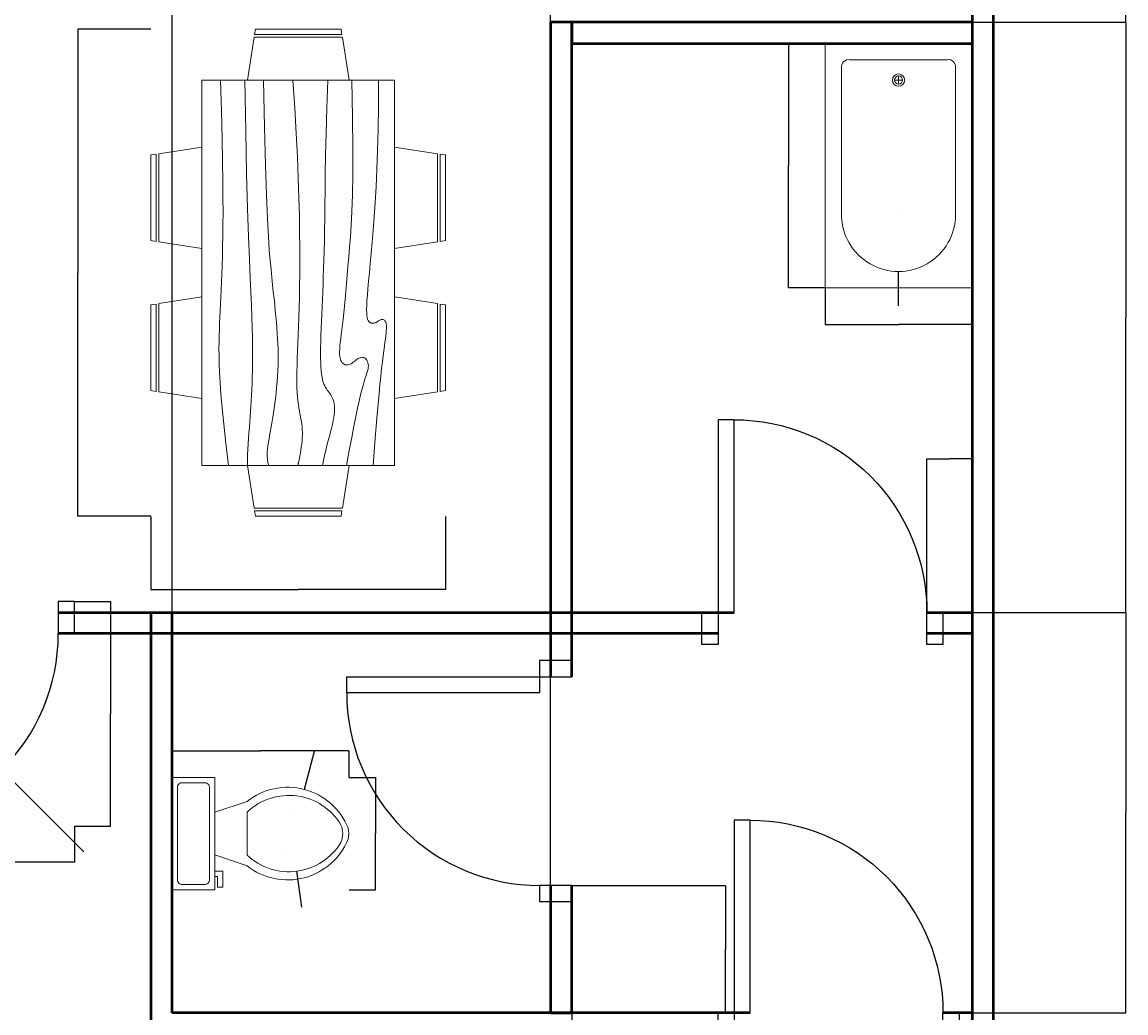
# Model space of a CAD drawing. Units: millimetres. Extents: x 756 to 17937, y 31 to 15590.
# Tile 4 of 6: x 7469 to 12704, y 7660 to 12361. Entities that reach past the tile are written whole.
import ezdxf

# ---------------------------------------------------------------- set-up
doc = ezdxf.new("R2010")
doc.units = ezdxf.units.MM
for name, color, linetype, lineweight in [('A-ANNO-DIMS', 2, 'Continuous', 18), ('A-DOOR', 3, 'Continuous', 25), ('A-FLOR-FIXT', 9, 'Continuous', 18), ('A-FURN', 8, 'Continuous', 18), ('A-WALL', 7, 'Continuous', 50)]:
    doc.layers.add(name, color=color, linetype=linetype, lineweight=lineweight)
doc.styles.get("Standard").update_dxf_attribs({"font": 'arial.ttf'})
doc.dimstyles.get("Standard").update_dxf_attribs({"dimtxt": 0.18, "dimasz": 0.18, "dimexe": 0.18, "dimexo": 0.0625, "dimgap": 0.09, "dimtad": 0, "dimtih": 1, "dimtoh": 1, "dimdec": 4, "dimzin": 0, "dimdsep": 46, "dimtxsty": 'Standard', "dimcen": 0.09, "dimadec": 0, "dimazin": 0, "dimtfac": 1, "dimtdec": 4, "dimtofl": 0, "dimtmove": 0, "dimatfit": 3, "dimfxl": 1, "dimtolj": 1, "dimtzin": 0, "dimarcsym": 0})

# ---------------------------------------------------------------- blocks, each defined once
blk = doc.blocks.new('Dining Set - 36 x 72 in.')
for p, q in [((-22, 27.5), (-22.1562, 26.50042)), ((-22, 27.5), (-6, 27.5)), ((-5.8437, 26.49966), (-6, 27.5)), ((6, 27.5), (5.8438, 26.50042)), ((6, 27.5), (22, 27.5)), ((22.1563, 26.49966), (22, 27.5)), ((-22.2343, 26.00059), (-23.4847, 17.99762)), ((-22.2304, 26), (-5.7608, 26)), ((-5.8416, 26.5), (-22.1534, 26.5)), ((-4.5152, 17.99762), (-5.7655, 25.99926)), ((5.7657, 26.00059), (4.5153, 17.99762)), ((5.7696, 26), (22.2392, 26)), ((22.1584, 26.5), (5.8466, 26.5)), ((23.4848, 17.99762), (22.2345, 25.99926)), ((36, 18), (-36, 18)), ((-36, 18), (-36, -18)), ((36, -18), (36, 18)), ((-44.0006, 8.23428), (-35.9976, 9.48474)), ((44.0006, 8.23428), (35.9976, 9.48474)), ((-45.5, 8), (-44.5004, 8.15617)), ((-45.5, 8), (-45.5, -8)), ((-44.5, -8.15843), (-44.5, 8.15338)), ((-44, 8.23041), (-44, -8.23915)), ((44, 8.23041), (44, -8.23915)), ((44.5, -8.15843), (44.5, 8.15338)), ((45.5, 8), (44.5005, 8.15617)), ((45.5, 8), (45.5, -8)), ((-44.4997, -8.15631), (-45.5, -8)), ((-35.9976, -9.48476), (-43.9993, -8.2345)), ((35.9976, -9.48476), (43.9993, -8.2345)), ((44.4997, -8.15631), (45.5, -8)), ((-36, -18), (36, -18)), ((-22.2343, -26.0006), (-23.4847, -17.99762)), ((-4.5152, -17.99762), (-5.7655, -25.99928)), ((5.7657, -26.0006), (4.5153, -17.99762)), ((23.4848, -17.99762), (22.2345, -25.99928)), ((-22.2304, -26), (-5.7608, -26)), ((-22, -27.5), (-22.1562, -26.50044)), ((-5.8416, -26.5), (-22.1534, -26.5)), ((-5.8437, -26.49967), (-6, -27.5)), ((5.7696, -26), (22.2392, -26)), ((6, -27.5), (5.8438, -26.50044)), ((22.1584, -26.5), (5.8466, -26.5)), ((22.1563, -26.49967), (22, -27.5)), ((-22, -27.5), (-6, -27.5)), ((6, -27.5), (22, -27.5))]:
    blk.add_line(p, q)
for points in [[(-36, 15), (-31.1772, 14.97754), (-26.8079, 14.91406), (-22.8538, 14.81543), (-19.276, 14.6875), (-16.0362, 14.53613), (-13.0957, 14.36718), (-10.4159, 14.18652), (-7.9583, 14), (-5.6904, 13.81315), (-3.6035, 13.63021), (-1.6954, 13.45508), (0.0365, 13.29166), (1.5945, 13.14388), (2.9811, 13.01562), (4.1988, 12.9108), (5.25, 12.83333), (6.1393, 12.78613), (6.8802, 12.76823), (7.4883, 12.77767), (7.9792, 12.8125), (8.3685, 12.87077), (8.6719, 12.95052), (8.9049, 13.0498), (9.0833, 13.16666), (9.2205, 13.29899), (9.3216, 13.44401), (9.3895, 13.59879), (9.4271, 13.76041), (9.4373, 13.92594), (9.4232, 14.09245), (9.3875, 14.257), (9.3333, 14.41666), (9.2638, 14.56917), (9.1836, 14.71484), (9.0975, 14.85465), (9.0104, 14.98958), (8.9272, 15.1206), (8.8529, 15.2487), (8.7922, 15.37483), (8.75, 15.5), (8.7305, 15.62467), (8.7344, 15.74739), (8.7617, 15.86621), (8.8125, 15.97916), (8.8867, 16.08431), (8.9844, 16.17968), (9.1055, 16.26334), (9.25, 16.33333), (9.4189, 16.38802), (9.6172, 16.42708), (9.8506, 16.45052), (10.125, 16.45833), (10.4463, 16.45052), (10.8203, 16.42708), (11.2529, 16.38802), (11.75, 16.33333), (12.3184, 16.26318), (12.9694, 16.17838), (13.7151, 16.07991), (14.5677, 15.96875), (15.5395, 15.84586), (16.6426, 15.71224), (17.8893, 15.56884), (19.2917, 15.41666), (20.859, 15.25667), (22.5879, 15.08984), (24.4721, 14.91715), (26.5052, 14.73958), (28.6809, 14.5581), (30.9929, 14.3737), (33.4347, 14.18733), (36, 14)], [(-36, 10), (-28.9766, 10.14274), (-23.1725, 10.20442), (-18.4241, 10.19775), (-14.5677, 10.13541), (-11.4399, 10.03011), (-8.877, 9.89453), (-6.7154, 9.74137), (-4.7917, 9.58333), (-2.9698, 9.43082), (-1.2246, 9.28515), (0.4415, 9.14534), (2.026, 9.01041), (3.5266, 8.87939), (4.9408, 8.7513), (6.266, 8.62516), (7.5, 8.5), (8.6411, 8.37549), (9.6914, 8.2539), (10.6538, 8.13818), (11.5312, 8.03125), (12.3267, 7.93603), (13.043, 7.85547), (13.6831, 7.79248), (14.25, 7.75), (14.7471, 7.7303), (15.1797, 7.73307), (15.5537, 7.75732), (15.875, 7.80208), (16.1494, 7.86637), (16.3828, 7.94922), (16.5811, 8.04964), (16.75, 8.16666), (16.8944, 8.29915), (17.0143, 8.44531), (17.1089, 8.60319), (17.1771, 8.77083), (17.218, 8.94629), (17.2305, 9.1276), (17.2137, 9.31282), (17.1667, 9.5), (17.0895, 9.6875), (16.987, 9.875), (16.8649, 10.0625), (16.7292, 10.25), (16.5856, 10.4375), (16.4401, 10.625), (16.2985, 10.8125), (16.1667, 11), (16.05, 11.18733), (15.9518, 11.3737), (15.8752, 11.5581), (15.8229, 11.73958), (15.798, 11.91715), (15.8034, 12.08984), (15.842, 12.25667), (15.9167, 12.41666), (16.0295, 12.56836), (16.1784, 12.70833), (16.3605, 12.83268), (16.5729, 12.9375), (16.8127, 13.01888), (17.0768, 13.07291), (17.3625, 13.0957), (17.6667, 13.08333), (17.9894, 13.03312), (18.3418, 12.94726), (18.7382, 12.82918), (19.1927, 12.68229), (19.7195, 12.51001), (20.3327, 12.31575), (21.0465, 12.10294), (21.875, 11.875), (22.8357, 11.63354), (23.959, 11.37304), (25.2786, 11.08618), (26.8282, 10.76562), (28.6414, 10.40405), (30.752, 9.99414), (33.1936, 9.52856), (36, 9)], [(-36, 5.5), (-30.7157, 5.3348), (-26.069, 5.20963), (-21.9946, 5.11767), (-18.4271, 5.05208), (-15.3009, 5.00602), (-12.5508, 4.97265), (-10.1112, 4.94515), (-7.9167, 4.91666), (-5.909, 4.88167), (-4.0586, 4.83984), (-2.3429, 4.79215), (-0.7396, 4.73958), (0.7739, 4.6831), (2.22, 4.6237), (3.6213, 4.56233), (5, 4.5), (6.373, 4.43782), (7.7344, 4.3776), (9.0723, 4.32129), (10.375, 4.27083), (11.6309, 4.22819), (12.8281, 4.19531), (13.9551, 4.17415), (15, 4.16666), (15.954, 4.17448), (16.819, 4.19791), (17.6001, 4.23698), (18.3021, 4.29166), (18.9299, 4.36198), (19.4883, 4.44791), (19.9823, 4.54948), (20.4167, 4.66666), (20.7969, 4.79899), (21.1302, 4.94401), (21.4245, 5.09879), (21.6875, 5.26041), (21.9271, 5.42594), (22.1511, 5.59245), (22.3672, 5.757), (22.5834, 5.91666), (22.8065, 6.06868), (23.0404, 6.21093), (23.2879, 6.34147), (23.5521, 6.45833), (23.8358, 6.55957), (24.142, 6.64323), (24.4735, 6.70735), (24.8334, 6.75), (25.2235, 6.76969), (25.642, 6.76692), (26.0858, 6.74267), (26.5521, 6.69791), (27.0379, 6.63362), (27.5404, 6.55078), (28.0565, 6.45036), (28.5834, 6.33333), (29.1242, 6.19987), (29.7071, 6.04687), (30.3661, 5.87044), (31.1354, 5.66666), (32.0493, 5.43164), (33.142, 5.16146), (34.4475, 4.85221), (36, 4.5)], [(-36, -1), (-30.7915, -0.6591), (-26.0195, -0.38216), (-21.6519, -0.16284), (-17.6563, 0.00521), (-14.0005, 0.12833), (-10.6523, 0.21289), (-7.5796, 0.26522), (-4.75, 0.29166), (-2.134, 0.29793), (0.2878, 0.28711), (2.5317, 0.26163), (4.6146, 0.22396), (6.5529, 0.17651), (8.3633, 0.12174), (10.0623, 0.06209), (11.6667, 0), (13.1899, -0.06201), (14.6341, -0.1211), (15.9982, -0.17432), (17.2813, -0.21875), (18.4823, -0.25147), (19.6003, -0.26953), (20.6343, -0.27002), (21.5834, -0.25), (22.4481, -0.20768), (23.2357, -0.14584), (23.9549, -0.06836), (24.6146, 0.02083), (25.2235, 0.11784), (25.7904, 0.21875), (26.3241, 0.31966), (26.8334, 0.41666), (27.3265, 0.50618), (27.8099, 0.58593), (28.2894, 0.65397), (28.7709, 0.70833), (29.2601, 0.74707), (29.763, 0.76823), (30.2855, 0.76985), (30.8334, 0.75), (31.4088, 0.70784), (31.9994, 0.64713), (32.589, 0.57275), (33.1615, 0.48958), (33.7008, 0.4025), (34.1908, 0.3164), (34.6153, 0.23616), (34.9584, 0.16666), (35.2099, 0.11165), (35.3848, 0.07031), (35.504, 0.04069), (35.5886, 0.02083), (35.6594, 0.00879), (35.7377, 0.0026), (35.8442, 0.00032), (36, 0)], [(-36, -6.5), (-27.1843, -6.31267), (-20.084, -6.1263), (-14.469, -5.9419), (-10.1094, -5.76042), (-6.7752, -5.58285), (-4.2363, -5.41016), (-2.2629, -5.24333), (-0.625, -5.08334), (0.8708, -4.93099), (2.2715, -4.78646), (3.5872, -4.64974), (4.8281, -4.52084), (6.0046, -4.39974), (7.127, -4.28646), (8.2053, -4.18099), (9.25, -4.08334), (10.2705, -3.99382), (11.2734, -3.91407), (12.2647, -3.84603), (13.25, -3.79167), (14.2354, -3.75293), (15.2266, -3.73177), (16.2295, -3.73015), (17.25, -3.75), (18.2912, -3.79248), (19.3451, -3.85547), (20.4009, -3.93604), (21.4479, -4.03125), (22.4754, -4.13819), (23.4727, -4.25391), (24.4289, -4.37549), (25.3334, -4.5), (26.1785, -4.62492), (26.9694, -4.74935), (27.7145, -4.87281), (28.4219, -4.99479), (29.1, -5.11483), (29.7572, -5.23242), (30.4016, -5.34709), (31.0417, -5.45834), (31.6837, -5.56437), (32.3262, -5.65821), (32.9658, -5.73153), (33.599, -5.77604), (34.2224, -5.78345), (34.8327, -5.74545), (35.4264, -5.65373), (36, -5.5)], [(-36, -10), (-26.4022, -9.81299), (-18.4675, -9.62891), (-11.9839, -9.45069), (-6.7396, -9.28125), (-2.5226, -9.12354), (0.8789, -8.98047), (3.6769, -8.85498), (6.0833, -8.75), (8.2767, -8.66765), (10.3021, -8.60677), (12.1712, -8.56543), (13.8958, -8.54167), (15.4876, -8.53353), (16.9583, -8.53907), (18.3197, -8.55632), (19.5834, -8.58334), (20.7616, -8.61841), (21.8685, -8.66081), (22.9188, -8.71004), (23.9271, -8.76563), (24.9081, -8.82707), (25.8763, -8.89388), (26.8465, -8.96558), (27.8334, -9.04167), (28.8474, -9.12118), (29.8828, -9.20117), (30.93, -9.27824), (31.9792, -9.34896), (33.0205, -9.40991), (34.0443, -9.45768), (35.0407, -9.48885), (36, -9.5)], [(-36, -14.5), (-30.0881, -14.33513), (-25.0332, -14.21224), (-20.7312, -14.12647), (-17.0781, -14.07292), (-13.97, -14.04671), (-11.3027, -14.04297), (-8.9724, -14.05681), (-6.875, -14.08334), (-4.9224, -14.11833), (-3.0905, -14.16016), (-1.3709, -14.20785), (0.2448, -14.26042), (1.7647, -14.3169), (3.1973, -14.3763), (4.5507, -14.43767), (5.8333, -14.5), (7.0554, -14.5621), (8.235, -14.62175), (9.3922, -14.67652), (10.5469, -14.72396), (11.7192, -14.76164), (12.929, -14.78711), (14.1965, -14.79794), (15.5417, -14.79167), (16.9933, -14.76424), (18.6152, -14.70508), (20.4804, -14.60197), (22.6615, -14.44271), (25.2312, -14.21509), (28.2624, -13.9069), (31.8277, -13.50594), (36, -13)]]:
    blk.add_lwpolyline(points)
blk = doc.blocks.new('Toilet - top')
for p, q in [((9.5, -6), (9.5, -2)), ((-8, -8.5), (-8, -8)), ((-7, -8), (-7, -9.5)), ((-4, -8), (-6, -14)), ((4, -8), (6, -14)), ((-10, -8.5), (-8, -8.5)), ((-10, -9.5), (-10, -8.5)), ((-7, -9.5), (-10, -9.5)), ((4, -14), (-4, -14))]:
    blk.add_line(p, q)
blk.add_lwpolyline([(10.5, -8), (10.5, 0), (-10.5, 0), (-10.5, -8)], close=True)
for points in [[(-9.5, -2), (-9.5, -6)], [(8.5, -1), (-8.5, -1)], [(-8.5, -7), (8.5, -7)]]:
    blk.add_lwpolyline(points)
for centre, radius, start, end in [((-8.62, -1.88), 0.884, 81.8699, 188.1301), ((8.62, -1.88), 0.884, 351.8699, 98.1301), ((-8.62, -6.12), 0.884, 171.8699, 278.1301), ((8.62, -6.12), 0.884, 261.8699, 8.1301), ((3.52, -21.58), 12.17, 141.4691, 247.9714), ((4.2, -21.82), 11.33, 136.3677, 238.9468), ((-3.52, -21.58), 12.17, 292.0284, 38.5307), ((-4.2, -21.82), 11.33, 301.053, 43.6321), ((0, -27.88), 4, 245.7318, 294.2682), ((0, -29), 4, 254.8605, 285.1395)]:
    blk.add_arc(centre, radius, start, end)
blk = doc.blocks.new('Bath Tub - 26 x 60 in.')
for p, q in [((8, -18), (10, -18)), ((9, -17), (9, -19))]:
    blk.add_line(p, q)
blk.add_lwpolyline([(0, -36), (0, 0), (60, 0), (60, -36)], close=True)
for points in [[(6, -4), (42, -4)], [(4, -30), (4, -6)], [(42, -32), (6, -32)]]:
    blk.add_lwpolyline(points)
for radius in [1.5, 1]:
    blk.add_circle((9, -18), radius)
for centre, radius, start, end in [((5.75, -5.75), 1.77, 81.8699, 188.1301), ((42, -18), 14, 270, 90), ((5.75, -30.25), 1.77, 171.8699, 278.1301)]:
    blk.add_arc(centre, radius, start, end)
blk = doc.blocks.new('DOOR-SINGLE-914')
for p, q in [((76.2, 1066.8), (0, 1066.8)), ((0, 1066.8), (0, 914.4)), ((76.2, 914.4), (76.2, 1066.8)), ((1143, 1066.8), (1066.8, 1066.8)), ((1066.8, 1066.8), (1066.8, 914.4)), ((1143, 914.4), (1143, 1066.8)), ((0, 914.4), (76.2, 914.4)), ((76.2, 914.4), (152.4, 914.4)), ((76.2, 0), (76.2, 914.4)), ((152.4, 914.4), (152.4, 0)), ((1066.8, 914.4), (1143, 914.4)), ((152.4, 0), (76.2, 0))]:
    blk.add_line(p, q)
blk.add_arc((152.4, 914.4), 914.4, 270, 0)
blk = doc.blocks.new('*D15')
at = {"layer": 'A-ANNO-DIMS', "color": 0, "lineweight": -2, "transparency": 16777216}
for p, q in [((6574.2, 8546.1), (6574.2, 8374.6)), ((7717.2, 8546.1), (7717.2, 8374.6)), ((6574.4, 8374.8), (7144.1, 8374.8)), ((7717, 8374.8), (7147.3, 8374.8))]:
    blk.add_line(p, q, dxfattribs=at)
at = {"layer": 'A-ANNO-DIMS', "color": 0, "transparency": 16777216}
for points in [[(6574.4, 8374.8), (6574.4, 8374.7), (6574.2, 8374.8)], [(7717, 8374.8), (7717, 8374.7), (7717.2, 8374.8)]]:
    blk.add_solid(points, dxfattribs=at)
at = {"layer": 'Defpoints', "color": 0, "transparency": 16777216}
for p in [(6574.2, 8546.2), (7717.2, 8546.2), (7717.2, 8374.8)]:
    blk.add_point(p, dxfattribs=at)
at = {"layer": 'A-ANNO-DIMS', "color": 0, "transparency": 16777216, "insert": (7145.7, 8374.8), "char_height": 0.18, "attachment_point": 5}
blk.add_mtext('\\A1;SINGLE DOOR 1143 TYP.', dxfattribs=at)
blk = doc.blocks.new('*D16')
at = {"layer": 'A-ANNO-DIMS', "color": 0, "lineweight": -2, "transparency": 16777216}
for p, q in [((7717.2, 9613), (7888.8, 9613)), ((7888.6, 9612.8), (7888.6, 9079.8)), ((7888.6, 8546.4), (7888.6, 9079.4)), ((7717.2, 8546.2), (7888.8, 8546.2))]:
    blk.add_line(p, q, dxfattribs=at)
at = {"layer": 'A-ANNO-DIMS', "color": 0, "transparency": 16777216}
for points in [[(7888.6, 9612.8), (7888.7, 9612.8), (7888.6, 9613)], [(7888.6, 8546.4), (7888.7, 8546.4), (7888.6, 8546.2)]]:
    blk.add_solid(points, dxfattribs=at)
at = {"layer": 'Defpoints', "color": 0, "transparency": 16777216}
for p in [(7717.2, 9613), (7888.6, 9613), (7717.2, 8546.2)]:
    blk.add_point(p, dxfattribs=at)
at = {"layer": 'A-ANNO-DIMS', "color": 0, "transparency": 16777216, "insert": (7888.6, 9079.6), "char_height": 0.18, "attachment_point": 5}
blk.add_mtext('\\A1;1067 TYP.', dxfattribs=at)
blk = doc.blocks.new('*D31')
at = {"layer": 'A-ANNO-DIMS', "color": 0, "lineweight": -2, "transparency": 16777216}
for p, q in [((8080.2, 12327.8), (7733.4, 12327.8)), ((7733.5, 12327.6), (7733.5, 11172.3)), ((7733.5, 10016.5), (7733.5, 11171.9)), ((8080.2, 10016.4), (7733.4, 10016.4))]:
    blk.add_line(p, q, dxfattribs=at)
at = {"layer": 'A-ANNO-DIMS', "color": 0, "transparency": 16777216}
for points in [[(7733.5, 12327.6), (7733.6, 12327.6), (7733.5, 12327.8)], [(7733.5, 10016.5), (7733.6, 10016.5), (7733.5, 10016.4)]]:
    blk.add_solid(points, dxfattribs=at)
at = {"layer": 'Defpoints', "color": 0, "transparency": 16777216}
for p in [(8080.2, 12327.8), (7733.5, 10016.4), (8080.2, 10016.4)]:
    blk.add_point(p, dxfattribs=at)
at = {"layer": 'A-ANNO-DIMS', "color": 0, "transparency": 16777216, "insert": (7733.5, 11172.1), "char_height": 0.18, "attachment_point": 5}
blk.add_mtext('\\A1;DINING SET 2311', dxfattribs=at)
blk = doc.blocks.new('*D32')
at = {"layer": 'A-ANNO-DIMS', "color": 0, "lineweight": -2, "transparency": 16777216}
for p, q in [((8080.2, 10016.3), (8080.2, 9669.5)), ((9477.2, 10016.3), (9477.2, 9669.5)), ((8080.4, 9669.7), (8778.4, 9669.7)), ((9477.1, 9669.7), (8779.1, 9669.7))]:
    blk.add_line(p, q, dxfattribs=at)
at = {"layer": 'A-ANNO-DIMS', "color": 0, "transparency": 16777216}
for points in [[(8080.4, 9669.7), (8080.4, 9669.6), (8080.2, 9669.7)], [(9477.1, 9669.7), (9477.1, 9669.6), (9477.2, 9669.7)]]:
    blk.add_solid(points, dxfattribs=at)
at = {"layer": 'Defpoints', "color": 0, "transparency": 16777216}
for p in [(8080.2, 10016.4), (9477.2, 10016.4), (9477.2, 9669.7)]:
    blk.add_point(p, dxfattribs=at)
at = {"layer": 'A-ANNO-DIMS', "color": 0, "transparency": 16777216, "insert": (8778.7, 9669.7), "char_height": 0.18, "attachment_point": 5}
blk.add_mtext('\\A1;1397', dxfattribs=at)
blk = doc.blocks.new('*D39')
at = {"layer": 'A-ANNO-DIMS', "color": 0, "lineweight": -2, "transparency": 16777216}
for p, q in [((11277.6, 12260.2), (11103.5, 12260.2)), ((11103.7, 12260), (11103.7, 11680.6)), ((11103.7, 11100.8), (11103.7, 11680.2)), ((11277.6, 11100.7), (11103.5, 11100.7))]:
    blk.add_line(p, q, dxfattribs=at)
at = {"layer": 'A-ANNO-DIMS', "color": 0, "transparency": 16777216}
for points in [[(11103.7, 12260), (11103.7, 12260), (11103.7, 12260.2)], [(11103.7, 11100.8), (11103.7, 11100.8), (11103.7, 11100.7)]]:
    blk.add_solid(points, dxfattribs=at)
at = {"layer": 'Defpoints', "color": 0, "transparency": 16777216}
for p in [(11277.6, 12260.2), (11103.7, 11100.7), (11277.6, 11100.7)]:
    blk.add_point(p, dxfattribs=at)
at = {"layer": 'A-ANNO-DIMS', "color": 0, "transparency": 16777216, "insert": (11103.7, 11680.4), "char_height": 0.18, "attachment_point": 5}
blk.add_mtext('\\A1;BATHTUB 1160', dxfattribs=at)
blk = doc.blocks.new('*D40')
at = {"layer": 'A-ANNO-DIMS', "color": 0, "lineweight": -2, "transparency": 16777216}
for p, q in [((11277.6, 11100.6), (11277.6, 10926.6)), ((11973.3, 11100.6), (11973.3, 10926.6)), ((11277.8, 10926.7), (11625.2, 10926.7)), ((11973.1, 10926.7), (11625.8, 10926.7))]:
    blk.add_line(p, q, dxfattribs=at)
at = {"layer": 'A-ANNO-DIMS', "color": 0, "transparency": 16777216}
for points in [[(11277.8, 10926.8), (11277.8, 10926.7), (11277.6, 10926.7)], [(11973.1, 10926.8), (11973.1, 10926.7), (11973.3, 10926.7)]]:
    blk.add_solid(points, dxfattribs=at)
at = {"layer": 'Defpoints', "color": 0, "transparency": 16777216}
for p in [(11277.6, 11100.7), (11973.3, 11100.7), (11973.3, 10926.7)]:
    blk.add_point(p, dxfattribs=at)
at = {"layer": 'A-ANNO-DIMS', "color": 0, "transparency": 16777216, "insert": (11625.5, 10926.7), "char_height": 0.18, "attachment_point": 5}
blk.add_mtext('\\A1;696', dxfattribs=at)
blk = doc.blocks.new('*D41')
at = {"layer": 'A-ANNO-DIMS', "color": 0, "lineweight": -2, "transparency": 16777216}
for p, q in [((8180.2, 8777.9), (8180.2, 8903.9)), ((8180.4, 8903.7), (8599.4, 8903.7)), ((9019.4, 8903.7), (8600.5, 8903.7)), ((9019.6, 8777.9), (9019.6, 8903.9))]:
    blk.add_line(p, q, dxfattribs=at)
at = {"layer": 'A-ANNO-DIMS', "color": 0, "transparency": 16777216}
for points in [[(8180.4, 8903.7), (8180.4, 8903.7), (8180.2, 8903.7)], [(9019.4, 8903.7), (9019.4, 8903.7), (9019.6, 8903.7)]]:
    blk.add_solid(points, dxfattribs=at)
at = {"layer": 'Defpoints', "color": 0, "transparency": 16777216}
for p in [(8180.2, 8903.7), (8180.2, 8777.8), (9019.6, 8777.8)]:
    blk.add_point(p, dxfattribs=at)
at = {"layer": 'A-ANNO-DIMS', "color": 0, "transparency": 16777216, "insert": (8599.9, 8903.7), "char_height": 0.18, "attachment_point": 5}
blk.add_mtext('\\A1;WC 839', dxfattribs=at)
blk = doc.blocks.new('*D42')
at = {"layer": 'A-ANNO-DIMS', "color": 0, "lineweight": -2, "transparency": 16777216}
for p, q in [((9019.7, 8777.8), (9145.7, 8777.8)), ((9145.5, 8777.6), (9145.5, 8511.3)), ((9145.5, 8244.6), (9145.5, 8510.9)), ((9019.7, 8244.4), (9145.7, 8244.4))]:
    blk.add_line(p, q, dxfattribs=at)
at = {"layer": 'A-ANNO-DIMS', "color": 0, "transparency": 16777216}
for points in [[(9145.5, 8777.6), (9145.5, 8777.6), (9145.5, 8777.8)], [(9145.5, 8244.6), (9145.5, 8244.6), (9145.5, 8244.4)]]:
    blk.add_solid(points, dxfattribs=at)
at = {"layer": 'Defpoints', "color": 0, "transparency": 16777216}
for p in [(9019.6, 8777.8), (9145.5, 8777.8), (9019.6, 8244.4)]:
    blk.add_point(p, dxfattribs=at)
at = {"layer": 'A-ANNO-DIMS', "color": 0, "transparency": 16777216, "insert": (9145.5, 8511.1), "char_height": 0.18, "attachment_point": 5}
blk.add_mtext('\\A1;533', dxfattribs=at)
blk = doc.blocks.new('*D50')
at = {"layer": 'A-ANNO-DIMS', "color": 0, "lineweight": -2, "transparency": 16777216}
for p, q in [((11974.2, 9560.2), (12703.5, 9560.2)), ((12703.4, 9560), (12703.4, 8610.4)), ((12703.4, 7660.4), (12703.4, 8610)), ((11974.2, 7660.2), (12703.5, 7660.2))]:
    blk.add_line(p, q, dxfattribs=at)
at = {"layer": 'A-ANNO-DIMS', "color": 0, "transparency": 16777216}
for points in [[(12703.3, 9560), (12703.4, 9560), (12703.4, 9560.2)], [(12703.3, 7660.4), (12703.4, 7660.4), (12703.4, 7660.2)]]:
    blk.add_solid(points, dxfattribs=at)
at = {"layer": 'Defpoints', "color": 0, "transparency": 16777216}
for p in [(11974.1, 9560.2), (11974.1, 7660.2), (12703.4, 7660.2)]:
    blk.add_point(p, dxfattribs=at)
at = {"layer": 'A-ANNO-DIMS', "color": 0, "transparency": 16777216, "insert": (12703.4, 8610.2), "char_height": 0.18, "attachment_point": 5}
blk.add_mtext('\\A1;1900', dxfattribs=at)
blk = doc.blocks.new('*D51')
at = {"layer": 'A-ANNO-DIMS', "color": 0, "lineweight": -2, "transparency": 16777216}
for p, q in [((11974.2, 12360.2), (12703.5, 12360.2)), ((12703.4, 12360), (12703.4, 10960.4)), ((12703.4, 9560.4), (12703.4, 10960)), ((11974.2, 9560.2), (12703.5, 9560.2))]:
    blk.add_line(p, q, dxfattribs=at)
at = {"layer": 'A-ANNO-DIMS', "color": 0, "transparency": 16777216}
for points in [[(12703.3, 12360), (12703.4, 12360), (12703.4, 12360.2)], [(12703.3, 9560.4), (12703.4, 9560.4), (12703.4, 9560.2)]]:
    blk.add_solid(points, dxfattribs=at)
at = {"layer": 'Defpoints', "color": 0, "transparency": 16777216}
for p in [(11974.1, 12360.2), (11974.1, 9560.2), (12703.4, 9560.2)]:
    blk.add_point(p, dxfattribs=at)
at = {"layer": 'A-ANNO-DIMS', "color": 0, "transparency": 16777216, "insert": (12703.4, 10960.2), "char_height": 0.18, "attachment_point": 5}
blk.add_mtext('\\A1;2800', dxfattribs=at)
blk = doc.blocks.new('*D52')
at = {"layer": 'A-ANNO-DIMS', "color": 0, "lineweight": -2, "transparency": 16777216}
for p, q in [((11974.2, 14760.2), (12703.5, 14760.2)), ((12703.4, 14760), (12703.4, 13560.4)), ((12703.4, 12360.4), (12703.4, 13560)), ((11974.2, 12360.2), (12703.5, 12360.2))]:
    blk.add_line(p, q, dxfattribs=at)
at = {"layer": 'A-ANNO-DIMS', "color": 0, "transparency": 16777216}
for points in [[(12703.3, 14760), (12703.4, 14760), (12703.4, 14760.2)], [(12703.3, 12360.4), (12703.4, 12360.4), (12703.4, 12360.2)]]:
    blk.add_solid(points, dxfattribs=at)
at = {"layer": 'Defpoints', "color": 0, "transparency": 16777216}
for p in [(11974.1, 14760.2), (11974.1, 12360.2), (12703.4, 12360.2)]:
    blk.add_point(p, dxfattribs=at)
at = {"layer": 'A-ANNO-DIMS', "color": 0, "transparency": 16777216, "insert": (12703.4, 13560.2), "char_height": 0.18, "attachment_point": 5}
blk.add_mtext('\\A1;2400', dxfattribs=at)
blk = doc.blocks.new('*D61')
at = {"layer": 'A-ANNO-DIMS', "color": 0, "lineweight": -2, "transparency": 16777216}
for p, q in [((8180.2, 7660.2), (8180.2, 15589.6)), ((8180.4, 15589.4), (9077.5, 15589.4)), ((9975.2, 15589.4), (9078.2, 15589.4)), ((9975.4, 7660.2), (9975.4, 15589.6))]:
    blk.add_line(p, q, dxfattribs=at)
at = {"layer": 'A-ANNO-DIMS', "color": 0, "transparency": 16777216}
for points in [[(8180.4, 15589.5), (8180.4, 15589.4), (8180.2, 15589.4)], [(9975.2, 15589.5), (9975.2, 15589.4), (9975.4, 15589.4)]]:
    blk.add_solid(points, dxfattribs=at)
at = {"layer": 'Defpoints', "color": 0, "transparency": 16777216}
for p in [(9975.4, 15589.4), (8180.2, 7660.2), (9975.4, 7660.2)]:
    blk.add_point(p, dxfattribs=at)
at = {"layer": 'A-ANNO-DIMS', "color": 0, "transparency": 16777216, "insert": (9077.8, 15589.4), "char_height": 0.18, "attachment_point": 5}
blk.add_mtext('\\A1;1795', dxfattribs=at)
blk = doc.blocks.new('*D62')
at = {"layer": 'A-ANNO-DIMS', "color": 0, "lineweight": -2, "transparency": 16777216}
for p, q in [((10075.4, 7660.1), (10075.4, 30.8)), ((11974.1, 7660.1), (11974.1, 30.8)), ((10075.6, 30.9), (11024.3, 30.9)), ((11973.9, 30.9), (11025.2, 30.9))]:
    blk.add_line(p, q, dxfattribs=at)
at = {"layer": 'A-ANNO-DIMS', "color": 0, "transparency": 16777216}
for points in [[(10075.6, 31), (10075.6, 30.9), (10075.4, 30.9)], [(11973.9, 31), (11973.9, 30.9), (11974.1, 30.9)]]:
    blk.add_solid(points, dxfattribs=at)
at = {"layer": 'Defpoints', "color": 0, "transparency": 16777216}
for p in [(10075.4, 7660.2), (11974.1, 7660.2), (11974.1, 30.9)]:
    blk.add_point(p, dxfattribs=at)
at = {"layer": 'A-ANNO-DIMS', "color": 0, "transparency": 16777216, "insert": (11024.7, 30.9), "char_height": 0.18, "attachment_point": 5}
blk.add_mtext('\\A1;1898.7', dxfattribs=at)
blk = doc.blocks.new('*D72')
at = {"layer": 'A-ANNO-DIMS', "color": 0, "lineweight": -2, "transparency": 16777216}
for p, q in [((11760, 9560.2), (11760, 10289.6)), ((11760.2, 10289.4), (11866.6, 10289.4)), ((11973.9, 10289.4), (11867.5, 10289.4)), ((11974.1, 9560.2), (11974.1, 10289.6))]:
    blk.add_line(p, q, dxfattribs=at)
at = {"layer": 'A-ANNO-DIMS', "color": 0, "transparency": 16777216}
for points in [[(11760.2, 10289.5), (11760.2, 10289.4), (11760, 10289.4)], [(11973.9, 10289.5), (11973.9, 10289.4), (11974.1, 10289.4)]]:
    blk.add_solid(points, dxfattribs=at)
at = {"layer": 'Defpoints', "color": 0, "transparency": 16777216}
for p in [(11974.1, 10289.4), (11760, 9560.2), (11974.1, 9560.2)]:
    blk.add_point(p, dxfattribs=at)
at = {"layer": 'A-ANNO-DIMS', "color": 0, "transparency": 16777216, "insert": (11867.1, 10289.4), "char_height": 0.18, "attachment_point": 5}
blk.add_mtext('\\A1;214.12', dxfattribs=at)
blk = doc.blocks.new('*D73')
at = {"layer": 'A-ANNO-DIMS', "color": 0, "lineweight": -2, "transparency": 16777216}
for p, q in [((10075.4, 8264.9), (10804.8, 8264.9)), ((10804.6, 8264.7), (10804.6, 7962.7)), ((10804.6, 7660.4), (10804.6, 7962.4)), ((10075.4, 7660.2), (10804.8, 7660.2))]:
    blk.add_line(p, q, dxfattribs=at)
at = {"layer": 'A-ANNO-DIMS', "color": 0, "transparency": 16777216}
for points in [[(10804.6, 8264.7), (10804.7, 8264.7), (10804.6, 8264.9)], [(10804.6, 7660.4), (10804.7, 7660.4), (10804.6, 7660.2)]]:
    blk.add_solid(points, dxfattribs=at)
at = {"layer": 'Defpoints', "color": 0, "transparency": 16777216}
for p in [(10075.4, 8264.9), (10075.4, 7660.2), (10804.6, 7660.2)]:
    blk.add_point(p, dxfattribs=at)
at = {"layer": 'A-ANNO-DIMS', "color": 0, "transparency": 16777216, "insert": (10804.6, 7962.6), "char_height": 0.18, "attachment_point": 5}
blk.add_mtext('\\A1;604.7', dxfattribs=at)
blk = doc.blocks.new('*D78')
at = {"layer": 'A-ANNO-DIMS', "color": 0, "lineweight": -2, "transparency": 16777216}
for p, q in [((6726.5, 9460.6), (6726.7, 9460.6)), ((6726.6, 9460.5), (6726.6, 9460.7)), ((7761.1, 8426.1), (7373.3, 8813.9)), ((7761.3, 8426.1), (7761.1, 8426.1))]:
    blk.add_line(p, q, dxfattribs=at)
at = {"layer": 'A-ANNO-DIMS', "color": 0, "transparency": 16777216}
blk.add_solid([(7373.3, 8813.9), (7373.3, 8813.9), (7373.2, 8814)], dxfattribs=at)
at = {"layer": 'Defpoints', "color": 0, "transparency": 16777216}
for p in [(6726.6, 9460.6), (7373.2, 8814)]:
    blk.add_point(p, dxfattribs=at)
at = {"layer": 'A-ANNO-DIMS', "color": 0, "transparency": 16777216, "insert": (7762, 8426.1), "char_height": 0.18, "attachment_point": 5}
blk.add_mtext('\\A1;5X R914.4', dxfattribs=at)
blk = doc.blocks.new('*D82')
at = {"layer": 'A-ANNO-DIMS', "color": 0, "lineweight": -2, "transparency": 16777216}
for p, q in [((8854, 8900), (8807, 8720.8)), ((8854.2, 8900), (8854, 8900)), ((8728.3, 8421.7), (8728.5, 8421.7)), ((8728.4, 8421.6), (8728.4, 8421.8))]:
    blk.add_line(p, q, dxfattribs=at)
at = {"layer": 'A-ANNO-DIMS', "color": 0, "transparency": 16777216}
blk.add_solid([(8806.9, 8720.8), (8807, 8720.8), (8806.9, 8720.7)], dxfattribs=at)
at = {"layer": 'Defpoints', "color": 0, "transparency": 16777216}
for p in [(8806.9, 8720.7), (8728.4, 8421.7)]:
    blk.add_point(p, dxfattribs=at)
at = {"layer": 'A-ANNO-DIMS', "color": 0, "transparency": 16777216, "insert": (8854.9, 8900), "char_height": 0.18, "attachment_point": 5}
blk.add_mtext('\\A1;2X R309.1', dxfattribs=at)
blk = doc.blocks.new('*D83')
at = {"layer": 'A-ANNO-DIMS', "color": 0, "lineweight": -2, "transparency": 16777216}
for p, q in [((8734.3, 8617.8), (8734.5, 8617.8)), ((8734.4, 8617.7), (8734.4, 8617.9)), ((8795.7, 8161.5), (8772.8, 8332.4)), ((8795.9, 8161.5), (8795.7, 8161.5))]:
    blk.add_line(p, q, dxfattribs=at)
at = {"layer": 'A-ANNO-DIMS', "color": 0, "transparency": 16777216}
blk.add_solid([(8772.8, 8332.4), (8772.7, 8332.4), (8772.7, 8332.6)], dxfattribs=at)
at = {"layer": 'Defpoints', "color": 0, "transparency": 16777216}
for p in [(8734.4, 8617.8), (8772.7, 8332.6)]:
    blk.add_point(p, dxfattribs=at)
at = {"layer": 'A-ANNO-DIMS', "color": 0, "transparency": 16777216, "insert": (8796.7, 8161.5), "char_height": 0.18, "attachment_point": 5}
blk.add_mtext('\\A1;2X R287.76', dxfattribs=at)
blk = doc.blocks.new('*D84')
at = {"layer": 'A-ANNO-DIMS', "color": 0, "lineweight": -2, "transparency": 16777216}
for p, q in [((11625.4, 11448.5), (11625.6, 11448.5)), ((11625.5, 11448.4), (11625.5, 11448.6)), ((11625.5, 11015.6), (11625.5, 11177.8)), ((11625.3, 11015.6), (11625.5, 11015.6))]:
    blk.add_line(p, q, dxfattribs=at)
at = {"layer": 'A-ANNO-DIMS', "color": 0, "transparency": 16777216}
blk.add_solid([(11625.4, 11177.8), (11625.5, 11177.8), (11625.5, 11178)], dxfattribs=at)
at = {"layer": 'Defpoints', "color": 0, "transparency": 16777216}
for p in [(11625.5, 11448.5), (11625.5, 11178)]:
    blk.add_point(p, dxfattribs=at)
at = {"layer": 'A-ANNO-DIMS', "color": 0, "transparency": 16777216, "insert": (11624.7, 11015.6), "char_height": 0.18, "attachment_point": 5}
blk.add_mtext('\\A1;R270.55', dxfattribs=at)

msp = doc.modelspace()

# ---------------------------------------------------------------- linework, layer by layer
at = {"layer": 'A-WALL'}
for p, q in [((11974.114, 14860.181), (11974.114, 12360.181)), ((12074.114, 14760.181), (12074.114, 7560.16)), ((11974.114, 12360.181), (9975.382, 12360.181)), ((9975.382, 12360.181), (9975.382, 9255.527)), ((10075.382, 12360.181), (10075.382, 12260.181)), ((10075.382, 9255.527), (10075.382, 12360.181)), ((11974.114, 12360.181), (11974.114, 9160.181)), ((10075.382, 12260.181), (11974.114, 12260.181)), ((7640.985, 9560.181), (10845.592, 9560.181)), ((8080.23, 9560.181), (8080.23, 7660.181)), ((8180.23, 7660.181), (8180.23, 9560.181)), ((11759.992, 9560.181), (11974.114, 9560.181)), ((11974.114, 9560.181), (11974.114, 9460.181)), ((10769.392, 9460.181), (7640.985, 9460.181)), ((11974.114, 9460.181), (11759.992, 9460.181)), ((11974.114, 9160.181), (11974.114, 7660.181)), ((9975.382, 8264.927), (9975.382, 7660.181)), ((10075.382, 7660.181), (10075.382, 8264.927)), ((8080.23, 7660.181), (8080.23, 7560.181)), ((10921.792, 7660.181), (8180.23, 7660.181)), ((9975.382, 7660.181), (10075.382, 7660.181)), ((11974.114, 7660.181), (11836.192, 7660.181)), ((11974.114, 7660.181), (11974.114, 7560.181))]:
    msp.add_line(p, q, dxfattribs=at)

# ---------------------------------------------------------------- block references
at = {"layer": 'A-DOOR', "extrusion": (0, 0, -1), "zscale": -1, "rotation": 180}
for p in [(-10693.191, 10474.581), (-10769.391, 8574.581)]:
    msp.add_blockref('DOOR-SINGLE-914', p, dxfattribs=at)
at = {"layer": 'A-DOOR'}
msp.add_blockref('DOOR-SINGLE-914', (6574.185, 8546.202), dxfattribs=at)
at = {"layer": 'A-DOOR', "rotation": 270}
msp.add_blockref('DOOR-SINGLE-914', (9008.581, 9331.727), dxfattribs=at)
at = {"layer": 'A-FLOR-FIXT'}
for name, p, xscale, yscale, zscale, rotation in [('Bath Tub - 26 x 60 in.', (11973.325, 12260.181), 19.32528847577517, 19.32528847577517, 19.32528847577517, 270), ('Toilet - top', (8180.23, 8511.108), 25.4, 25.4, 25.4, 90)]:
    msp.add_blockref(name, p, dxfattribs=dict(at, xscale=xscale, yscale=yscale, zscale=zscale, rotation=rotation))
at = {"layer": 'A-FURN', "xscale": 25.4, "yscale": 25.4, "zscale": 25.4, "rotation": 270}
msp.add_blockref('Dining Set - 36 x 72 in.', (8778.744, 11172.069), dxfattribs=at)

# ---------------------------------------------------------------- dimensions: what is measured, and where the dimension line sits
at = {"layer": 'A-ANNO-DIMS'}
for base, p1, p2, override, picture, middle in [((9975.382, 15589.431), (8180.23, 7660.181), (9975.382, 7660.181), {"dimdec": 0, "dimlfac": 1, "dimrnd": 0, "dimzin": 0, "dimdsep": 46, "dimlunit": 2}, '*D61', (9077.806, 15589.431)), ((11973.325, 10926.736), (11277.615, 11100.663), (11973.325, 11100.663), {"dimdec": 0, "dimlfac": 1, "dimrnd": 0, "dimzin": 0, "dimdsep": 46, "dimlunit": 2}, '*D40', (11625.47, 10926.736)), ((9477.244, 9669.659), (8080.244, 10016.369), (9477.244, 10016.369), {"dimdec": 0, "dimlfac": 1, "dimrnd": 0, "dimzin": 0, "dimdsep": 46, "dimlunit": 2}, '*D32', (8778.744, 9669.659)), ((11974.114, 30.931), (10075.382, 7660.181), (11974.114, 7660.181), {"dimdec": 1, "dimlfac": 1, "dimrnd": 0, "dimzin": 0, "dimdsep": 46, "dimlunit": 2}, '*D62', (11024.748, 30.931))]:
    dim = msp.add_linear_dim(base=base, p1=p1, p2=p2, dimstyle='Standard', override=override, dxfattribs=at)
    dim.commit()
    dim.dimension.update_dxf_attribs({"geometry": picture, "text_midpoint": middle})
for base, p1, p2, angle, override, picture, middle in [((12703.364, 12360.181), (11974.114, 14760.181), (11974.114, 12360.181), 270, {"dimdec": 0, "dimlfac": 1, "dimrnd": 0, "dimzin": 0, "dimdsep": 46, "dimlunit": 2}, '*D52', (12703.364, 13560.181)), ((12703.364, 9560.181), (11974.114, 12360.181), (11974.114, 9560.181), 270, {"dimdec": 0, "dimlfac": 1, "dimrnd": 0, "dimzin": 0, "dimdsep": 46, "dimlunit": 2}, '*D51', (12703.364, 10960.181)), ((11974.114, 10289.431), (11759.992, 9560.181), (11974.114, 9560.181), 0, {"dimdec": 2, "dimlfac": 1, "dimrnd": 0, "dimzin": 0, "dimdsep": 46, "dimlunit": 2}, '*D72', (11867.053, 10289.431)), ((12703.364, 7660.181), (11974.114, 9560.181), (11974.114, 7660.181), 270, {"dimdec": 0, "dimlfac": 1, "dimrnd": 0, "dimzin": 0, "dimdsep": 46, "dimlunit": 2}, '*D50', (12703.364, 8610.181)), ((9145.511, 8777.808), (9019.605, 8244.408), (9019.605, 8777.808), 90, {"dimdec": 0, "dimlfac": 1, "dimrnd": 0, "dimzin": 0, "dimdsep": 46, "dimlunit": 2}, '*D42', (9145.511, 8511.108)), ((10804.632, 7660.181), (10075.382, 8264.927), (10075.382, 7660.181), 270, {"dimdec": 1, "dimlfac": 1, "dimrnd": 0, "dimzin": 0, "dimdsep": 46, "dimlunit": 2}, '*D73', (10804.632, 7962.554))]:
    dim = msp.add_linear_dim(base=base, p1=p1, p2=p2, angle=angle, dimstyle='Standard', override=override, dxfattribs=at)
    dim.commit()
    dim.dimension.update_dxf_attribs({"geometry": picture, "text_midpoint": middle})
for base, p1, p2, angle, text, picture, middle in [((7733.534, 10016.369), (8080.244, 12327.769), (8080.244, 10016.369), 270, 'DINING SET <>', '*D31', (7733.534, 11172.069)), ((11103.687, 11100.663), (11277.615, 12260.181), (11277.615, 11100.663), 270, 'BATHTUB <>', '*D39', (11103.687, 11680.422)), ((7888.635, 9613.002), (7717.185, 8546.202), (7717.185, 9613.002), 90, '<> TYP.', '*D16', (7888.635, 9079.602)), ((8180.23, 8903.715), (9019.605, 8777.808), (8180.23, 8777.808), 180, 'WC <>', '*D41', (8599.917, 8903.715))]:
    dim = msp.add_linear_dim(base=base, p1=p1, p2=p2, angle=angle, text=text, dimstyle='Standard', override={"dimdec": 0, "dimlfac": 1, "dimrnd": 0, "dimzin": 0, "dimdsep": 46, "dimlunit": 2}, dxfattribs=at)
    dim.commit()
    dim.dimension.update_dxf_attribs({"geometry": picture, "text_midpoint": middle})
dim = msp.add_radius_dim(center=(11625.47, 11448.518), mpoint=(11625.47, 11177.964), dimstyle='Standard', override={"dimdec": 2, "dimlfac": 1, "dimrnd": 0, "dimzin": 0, "dimdsep": 46, "dimlunit": 2}, dxfattribs=at)
dim.commit()
dim.dimension.update_dxf_attribs({"geometry": '*D84', "text_midpoint": (11624.74, 11015.632), "dimtype": 164})
for center, mpoint, text, override, picture, middle in [((6726.585, 9460.602), (7373.164, 8814.024), '5X <>', {"dimdec": 1, "dimlfac": 1, "dimrnd": 0, "dimzin": 0, "dimdsep": 46, "dimlunit": 2}, '*D78', (7761.964, 8426.077)), ((8728.374, 8421.713), (8806.916, 8720.661), '2X <>', {"dimdec": 1, "dimlfac": 1, "dimrnd": 0, "dimzin": 0, "dimdsep": 46, "dimlunit": 2}, '*D82', (8854.879, 8900.03)), ((8734.392, 8617.787), (8772.736, 8332.592), '2X <>', {"dimdec": 2, "dimlfac": 1, "dimrnd": 0, "dimzin": 0, "dimdsep": 46, "dimlunit": 2}, '*D83', (8796.667, 8161.475))]:
    dim = msp.add_radius_dim(center=center, mpoint=mpoint, text=text, dimstyle='Standard', override=override, dxfattribs=at)
    dim.commit()
    dim.dimension.update_dxf_attribs({"geometry": picture, "text_midpoint": middle, "dimtype": 164})
dim = msp.add_linear_dim(base=(7717.185, 8374.752), p1=(6574.185, 8546.202), p2=(7717.185, 8546.202), text='SINGLE DOOR <> TYP.', dimstyle='Standard', override={"dimdec": 0, "dimlfac": 1, "dimrnd": 0, "dimzin": 0, "dimdsep": 46, "dimlunit": 2}, dxfattribs=at)
dim.commit()
dim.dimension.update_dxf_attribs({"geometry": '*D15', "text_midpoint": (7145.685, 8374.752)})

doc.saveas('drawing.dxf')
